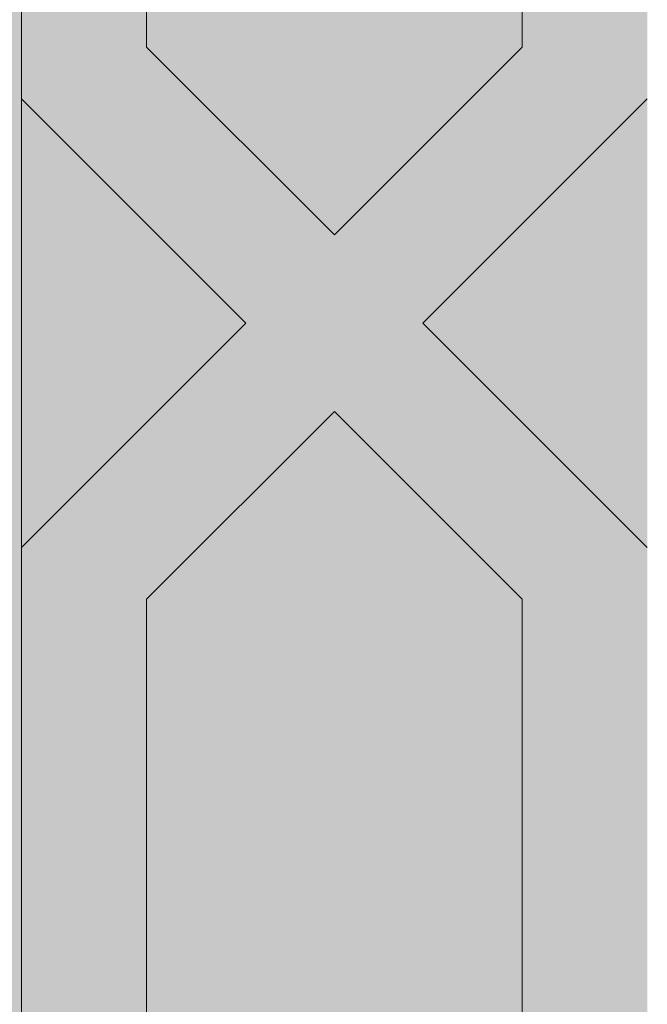
# Model space of a CAD drawing. Units: inches. Extents: x 844 to 2234, y 346 to 1084.
# Tile 70 of 93: x 1997.478 to 1998.757, y 694.327 to 696.335. Entities that reach past the tile are written whole.
import ezdxf

# ---------------------------------------------------------------- set-up
doc = ezdxf.new("R2010")
doc.units = ezdxf.units.IN
doc.header["$MEASUREMENT"] = 0
for name, color, linetype, lineweight in [('A-ANNO-DIMS', 2, 'Continuous', 18), ('furniture', 8, 'Continuous', 18), ('RA-AP-01$0$INT', 35, 'Continuous', 5)]:
    doc.layers.add(name, color=color, linetype=linetype, lineweight=lineweight)
doc.layers.add('RA-AP-01$0$FURN', color=3, linetype='Continuous')
doc.styles.get("Standard").update_dxf_attribs({"font": 'arial.ttf'})
doc.dimstyles.get("Standard").update_dxf_attribs({"dimtxt": 6, "dimasz": 3, "dimexe": 0.18, "dimexo": 0.0625, "dimgap": 0.09, "dimtad": 0, "dimtih": 1, "dimtoh": 1, "dimdec": 1, "dimzin": 0, "dimdsep": 46, "dimlunit": 3, "dimtxsty": 'Standard', "dimblk": 'ARCHTICK', "dimcen": 0.09, "dimadec": 0, "dimazin": 0, "dimtfac": 1, "dimtdec": 1, "dimtofl": 0, "dimtmove": 0, "dimatfit": 3, "dimfxl": 1, "dimtolj": 1, "dimtzin": 0, "dimarcsym": 0})

# ---------------------------------------------------------------- blocks, each defined once
blk = doc.blocks.new('A$C18D01794')
at = {"layer": 'RA-AP-01$0$INT'}
h = blk.add_hatch(color=256, dxfattribs=at)
h.paths.add_polyline_path([(4.355206456958071, -6.156712009588037), (4.355206456958071, -8.056712009588038), (5.455206456958072, -8.056712009588038), (5.455206456958072, -6.156712009588037)])
h.paths.add_polyline_path([(4.405206456958072, -8.006712009588039), (4.405206456958072, -6.206712009588038), (5.405206456958072, -6.206712009588038), (5.405206456958072, -8.006712009588039)], flags=16)
h = blk.add_hatch(color=256, dxfattribs=at)
h.paths.add_polyline_path([(4.469348592586677, -7.07085414521094), (4.505206456958073, -7.03499628085108), (4.505206456958071, -7.106712009593861)])
h.paths.add_polyline_path([(4.455206456960671, -7.084996280832395), (4.476922185709333, -7.106712009588038), (4.433490728198045, -7.106712009588038)])
h.paths.add_polyline_path([(4.405206456958073, -7.034996280813718), (4.441064321339218, -7.070854145206393), (4.40520645695807, -7.106712009576003)])
h.paths.add_polyline_path([(4.425206456989053, -6.911460746921742), (4.455206456990736, -6.881460746929706), (4.485206456989055, -6.911460746937677), (4.48520645696979, -7.026712009590022), (4.455206456965227, -7.056712009584936), (4.425206456969784, -7.026712009579853)])
h.paths.add_polyline_path([(4.505206456958073, -6.831460746955388), (4.505206456958071, -6.903176475661116), (4.469348592616738, -6.867318611308251)])
h.paths.add_polyline_path([(4.425206456964688, -6.707925213036777), (4.455206456964794, -6.677925213027025), (4.485206456964689, -6.707925213017265), (4.485206456983951, -6.823176475683938), (4.455206456990736, -6.853176475686799), (4.425206456983956, -6.823176475689667)])
h.paths.add_polyline_path([(4.425206456974126, -6.504389679118949), (4.455206456959092, -6.474389679124341), (4.485206456974132, -6.504389679129721), (4.485206456993396, -6.619640941768059), (4.45520645699153, -6.649640941779566), (4.425206456993394, -6.619640941791077)])
h.paths.add_polyline_path([(4.46934859260189, -6.663783077416661), (4.505206456958071, -6.627925213048953), (4.505206456958073, -6.699640941761311)])
h.paths.add_polyline_path([(4.405206456958073, -6.627925213005104), (4.441064321354427, -6.663783077389926), (4.405206456958072, -6.699640941797813)])
h.paths.add_polyline_path([(4.405206456958072, -6.424389679139403), (4.441064321333084, -6.460247543502882), (4.405206456958072, -6.496105407889427)])
h.paths.add_polyline_path([(4.469348592580547, -6.460247543498336), (4.505206456958071, -6.424389679109282), (4.505206456958071, -6.496105407864332)])
h.paths.add_polyline_path([(4.425206456957888, -6.300854145208262), (4.45520645695415, -6.270854145221655), (4.485206456959507, -6.300854145217359), (4.48520645695824, -6.416105407863534), (4.455206456954537, -6.44610540787688), (4.425206456957888, -6.416105407889874)])
h.paths.add_polyline_path([(4.425206456957888, -6.226712009591025), (4.471064321332215, -6.226712009591025), (4.425206456957888, -6.272569873980103)])
h.paths.add_polyline_path([(4.499348592575121, -6.226712009591029), (4.636064321343707, -6.226712009591025), (4.666064321342317, -6.256712009589254), (4.636064321340932, -6.286712009591028), (4.499348592588945, -6.286712009591028), (4.469348592591685, -6.256712009584116)])
h.paths.add_polyline_path([(4.680206456964641, -6.270854145214393), (4.716064321337824, -6.306712009588038), (4.644348592591454, -6.306712009588038)])
h.paths.add_polyline_path([(4.644348592588108, -6.206712009588038), (4.716064321341167, -6.206712009588038), (4.680206456964637, -6.242569873964111)])
h.paths.add_polyline_path([(4.724348592586768, -6.226712009589824), (4.861064321340514, -6.226712009589824), (4.891064321340324, -6.256712009589255), (4.861064321340141, -6.286712009589827), (4.724348592587134, -6.286712009589821), (4.694348592586957, -6.256712009589254)])
h.paths.add_polyline_path([(4.905206456964143, -6.270854145212892), (4.941064321338827, -6.306712009588038), (4.869348592589457, -6.306712009588039)])
h.paths.add_polyline_path([(4.869348592586113, -6.206712009588038), (4.941064321342172, -6.206712009588038), (4.905206456964145, -6.242569873965612)])
h.paths.add_polyline_path([(4.949348592587774, -6.226712009589824), (5.086064321341521, -6.226712009589824), (5.116064321341329, -6.256712009589252), (5.08606432134115, -6.286712009589823), (4.949348592588145, -6.286712009589827), (4.919348592587961, -6.256712009589255)])
h.paths.add_polyline_path([(5.130206456963645, -6.270854145214393), (5.166064321336834, -6.306712009588038), (5.094348592590464, -6.306712009588038)])
h.paths.add_polyline_path([(5.094348592587119, -6.206712009588038), (5.166064321340178, -6.206712009588038), (5.130206456963651, -6.242569873964107)])
h.paths.add_polyline_path([(5.174348592584578, -6.226712009591027), (5.311064321353163, -6.226712009591027), (5.341064321336602, -6.256712009584116), (5.31106432133934, -6.286712009591028), (5.174348592587352, -6.286712009591028), (5.144348592585969, -6.256712009589254)])
h.paths.add_polyline_path([(5.325206456968778, -6.300854145217359), (5.355206456974136, -6.270854145221653), (5.385206456970396, -6.300854145208262), (5.385206456970396, -6.416105407889878), (5.355206456973747, -6.44610540787688), (5.325206456970044, -6.416105407863533)])
h.paths.add_polyline_path([(5.339348592596073, -6.226712009591029), (5.385206456970396, -6.226712009591025), (5.385206456970398, -6.272569873980105)])
h.paths.add_polyline_path([(5.325206456954155, -6.504389679129722), (5.355206456969194, -6.474389679124342), (5.38520645695416, -6.504389679118949), (5.385206456934896, -6.619640941791077), (5.355206456936758, -6.649640941779564), (5.325206456934888, -6.619640941768057)])
h.paths.add_polyline_path([(5.305206456958072, -6.424389679097139), (5.341064321347739, -6.460247543498338), (5.305206456958072, -6.496105407876472)])
h.paths.add_polyline_path([(5.369348592595204, -6.460247543502882), (5.40520645695807, -6.42438967915155), (5.405206456958072, -6.496105407877278)])
h.paths.add_polyline_path([(5.405206456958072, -6.627925213017245), (5.405206456958072, -6.69964094178567), (5.369348592573857, -6.663783077389926)])
h.paths.add_polyline_path([(5.305206456958072, -6.62792521303681), (5.341064321326393, -6.663783077416663), (5.305206456958072, -6.69964094177345)])
h.paths.add_polyline_path([(5.325206456963599, -6.707925213017267), (5.355206456963494, -6.677925213027021), (5.385206456963598, -6.707925213036775), (5.385206456944334, -6.823176475689665), (5.355206456937552, -6.853176475686797), (5.325206456944333, -6.823176475683936)])
h.paths.add_polyline_path([(5.305206456958072, -6.831460746943246), (5.341064321311551, -6.867318611308252), (5.305206456958072, -6.903176475673257)])
h.paths.add_polyline_path([(5.325206456939231, -6.911460746937672), (5.355206456937552, -6.881460746929707), (5.385206456939235, -6.911460746921742), (5.385206456958502, -7.026712009579853), (5.355206456963061, -7.056712009584934), (5.3252064569585, -7.026712009590026)])
h.paths.add_polyline_path([(5.404581768715993, -6.832085435167151, 0.001217816984214), (5.405206456958072, -6.832312009593747), (5.405206456958072, -6.90317647569123), (5.369348592563558, -6.867318611308251)])
h.paths.add_polyline_path([(5.36934859258907, -7.070854145206393), (5.40520645695807, -7.034996280825861), (5.405206456958072, -7.106712009563858)])
h.paths.add_polyline_path([(5.355206456967613, -7.084996280832394), (5.376922185730239, -7.106712009588038), (5.333490728218953, -7.106712009588036)])
h.paths.add_polyline_path([(5.30520645695807, -7.034996280838937), (5.341064321341609, -7.070854145210942), (5.305206456958074, -7.106712009606006)])
h = blk.add_hatch(color=256, dxfattribs=at)
h.paths.add_polyline_path([(4.505206456958071, -6.627925213048953), (4.46934859260189, -6.663783077416663), (4.505206456958071, -6.699640941761309), (4.505206456958071, -6.831460746955389), (4.469348592616735, -6.867318611308252), (4.505206456958071, -6.903176475661112), (4.505206456958071, -7.03499628085108), (4.469348592586679, -7.070854145210939), (4.505206456952245, -7.106712009588038), (4.476922185709333, -7.106712009588038), (4.455206456960671, -7.084996280832395), (4.433490728198047, -7.106712009588038), (4.405206456946033, -7.10671200958804), (4.441064321339216, -7.070854145206393), (4.40520645695807, -7.034996280813718), (4.405206456958072, -6.903176475703379), (4.441064321364728, -6.867318611308251), (4.40520645695807, -6.83146074691313), (4.40520645695807, -6.699640941797813), (4.441064321354429, -6.663783077389924), (4.405206456958072, -6.627925213005102), (4.405206456958072, -6.496105407889425), (4.441064321333084, -6.460247543502882), (4.405206456958072, -6.424389679139403), (4.405206456958072, -6.206712009588038), (4.644348592588106, -6.206712009588038), (4.680206456964639, -6.242569873964107), (4.716064321341165, -6.206712009588038), (4.869348592586113, -6.206712009588038), (4.905206456964143, -6.24256987396561), (4.941064321342174, -6.206712009588038), (5.094348592587118, -6.206712009588038), (5.130206456963649, -6.242569873964107), (5.166064321340178, -6.206712009588038), (5.405206456958072, -6.206712009588038), (5.405206456958072, -6.42438967915155), (5.369348592595202, -6.46024754350288), (5.40520645695807, -6.49610540787728), (5.40520645695807, -6.627925213017247), (5.369348592573859, -6.663783077389926), (5.40520645695807, -6.699640941785666), (5.40520645695807, -6.831460746925273), (5.36934859256356, -6.867318611308252), (5.405206456958072, -6.90317647569123), (5.405206456958072, -7.034996280825859), (5.369348592589068, -7.070854145206395), (5.405206456982249, -7.106712009588038), (5.376922185730244, -7.106712009588038), (5.355206456967613, -7.084996280832397), (5.333490728218955, -7.106712009588036), (5.305206456976043, -7.106712009588035), (5.341064321341609, -7.07085414521094), (5.305206456958072, -7.034996280838935), (5.305206456958072, -6.90317647567326), (5.34106432131155, -6.867318611308252), (5.305206456958072, -6.831460746943244), (5.30520645695807, -6.699640941773452), (5.341064321326395, -6.663783077416663), (5.305206456958072, -6.627925213036814), (5.305206456958072, -6.496105407876472), (5.341064321347738, -6.46024754349834), (5.305206456958072, -6.424389679097137), (5.30520645695807, -6.306712009588038), (5.166064321336834, -6.306712009588038), (5.130206456963647, -6.270854145214393), (5.094348592590464, -6.306712009588038), (4.941064321338827, -6.306712009588036), (4.905206456964145, -6.270854145212892), (4.869348592589459, -6.306712009588038), (4.716064321337822, -6.306712009588036), (4.680206456964641, -6.270854145214393), (4.644348592591453, -6.306712009588038), (4.505206456958071, -6.306712009588038), (4.505206456958071, -6.424389679109282), (4.469348592580545, -6.460247543498338), (4.505206456958071, -6.496105407864328)])
h.paths.add_polyline_path([(4.485206456974132, -6.504389679129722), (4.45520645695909, -6.474389679124341), (4.425206456974128, -6.504389679118945), (4.425206456993394, -6.619640941791079), (4.45520645699153, -6.649640941779566), (4.485206456993396, -6.619640941768059)], flags=16)
h.paths.add_polyline_path([(4.455206456954537, -6.44610540787688), (4.485206456958242, -6.416105407863534), (4.48520645695951, -6.30085414521736), (4.45520645695415, -6.270854145221653), (4.425206456957888, -6.300854145208264), (4.425206456957888, -6.41610540788988)], flags=16)
h.paths.add_polyline_path([(4.455206456964794, -6.677925213027025), (4.42520645696469, -6.707925213036777), (4.425206456983954, -6.82317647568967), (4.455206456990734, -6.853176475686797), (4.485206456983953, -6.823176475683936), (4.485206456964687, -6.707925213017265)], flags=16)
h.paths.add_polyline_path([(4.499348592588947, -6.286712009591028), (4.636064321340932, -6.286712009591028), (4.666064321342317, -6.256712009589254), (4.636064321343707, -6.226712009591027), (4.499348592575121, -6.226712009591029), (4.469348592591685, -6.256712009584118)], flags=16)
h.paths.add_polyline_path([(4.425206456957888, -6.272569873980103), (4.471064321332215, -6.226712009591025), (4.425206456957888, -6.226712009591025)], flags=16)
h.paths.add_polyline_path([(4.455206456990734, -6.881460746929709), (4.425206456989053, -6.91146074692174), (4.425206456969784, -7.026712009579853), (4.455206456965226, -7.056712009584932), (4.485206456969787, -7.026712009590026), (4.485206456989053, -6.911460746937672)], flags=16)
h.paths.add_polyline_path([(4.72434859258714, -6.286712009589821), (4.861064321340141, -6.286712009589829), (4.891064321340324, -6.256712009589254), (4.861064321340513, -6.226712009589823), (4.724348592586768, -6.226712009589823), (4.694348592586956, -6.256712009589254)], flags=16)
h.paths.add_polyline_path([(4.919348592587961, -6.256712009589254), (4.949348592588145, -6.286712009589827), (5.08606432134115, -6.286712009589823), (5.116064321341327, -6.256712009589254), (5.086064321341519, -6.226712009589824), (4.949348592587774, -6.226712009589824)], flags=16)
h.paths.add_polyline_path([(5.144348592585967, -6.256712009589254), (5.174348592587358, -6.286712009591028), (5.311064321339338, -6.286712009591028), (5.3410643213366, -6.256712009584118), (5.311064321353163, -6.226712009591029), (5.174348592584576, -6.226712009591027)], flags=16)
h.paths.add_polyline_path([(5.32520645693489, -6.619640941768055), (5.355206456936755, -6.649640941779566), (5.385206456934894, -6.619640941791079), (5.38520645695416, -6.504389679118949), (5.355206456969194, -6.474389679124341), (5.325206456954153, -6.504389679129724)], flags=16)
h.paths.add_polyline_path([(5.325206456970042, -6.416105407863534), (5.355206456973747, -6.44610540787688), (5.385206456970398, -6.416105407889876), (5.385206456970398, -6.30085414520826), (5.355206456974136, -6.270854145221653), (5.325206456968778, -6.30085414521736)], flags=16)
h.paths.add_polyline_path([(5.325206456963599, -6.707925213017265), (5.325206456944333, -6.823176475683936), (5.355206456937552, -6.853176475686797), (5.385206456944332, -6.823176475689667), (5.385206456963596, -6.707925213036773), (5.355206456963492, -6.677925213027027)], flags=16)
h.paths.add_polyline_path([(5.32520645693923, -6.911460746937674), (5.3252064569585, -7.026712009590026), (5.355206456963062, -7.056712009584934), (5.3852064569585, -7.026712009579853), (5.385206456939234, -6.911460746921738), (5.355206456937552, -6.881460746929707)], flags=16)
h.paths.add_polyline_path([(5.339348592596071, -6.226712009591029), (5.385206456970398, -6.272569873980103), (5.385206456970396, -6.226712009591027)], flags=16)
for p, q in [((5.32520645693489, -6.619640941768059), (5.325206456954155, -6.504389679129722)), ((5.385206456934892, -6.619640941791081), (5.385206456954159, -6.504389679118947)), ((5.32520645693489, -6.619640941768059), (5.355206456936756, -6.649640941779566)), ((5.385206456934892, -6.619640941791081), (5.355206456936756, -6.649640941779566)), ((5.305206456939818, -6.627925213018556), (5.341064321310754, -6.663783077401021)), ((5.405206456939818, -6.627925213035499), (5.369348592558215, -6.663783077405568)), ((5.305206456959569, -6.699640941771955), (5.341064321342035, -6.663783077401022)), ((5.405206456959569, -6.699640941787167), (5.369348592589498, -6.663783077405566)), ((5.325206456963599, -6.707925213017265), (5.35520645696349, -6.677925213027025)), ((5.385206456963598, -6.707925213036777), (5.35520645696349, -6.677925213027025)), ((5.325206456944333, -6.823176475683936), (5.325206456963599, -6.707925213017265)), ((5.385206456944332, -6.823176475689667), (5.385206456963598, -6.707925213036777))]:
    blk.add_line(p, q, dxfattribs=at)
blk.add_lwpolyline([(5.405206456958072, -7.106712009588038), (5.405206456958072, -6.206712009588038)], dxfattribs=at)
blk = doc.blocks.new('A$C5D2F253E')
at = {"layer": 'RA-AP-01$0$FURN', "xscale": -0.7999999999883585, "yscale": 0.7999999999883585, "zscale": 0.8, "rotation": 90}
blk.add_blockref('A$C18D01794', (-5.687757199772477, 4.75791982714071), dxfattribs=at)
blk = doc.blocks.new('_ArchTick')
at = {"color": 0, "linetype": 'ByBlock', "const_width": 0.15}
blk.add_lwpolyline([(-0.5, -0.5), (0.5, 0.5)], dxfattribs=at)
blk = doc.blocks.new('*D121')
at = {"layer": 'A-ANNO-DIMS', "color": 0, "lineweight": -2, "transparency": 16777216}
for p, q in [((2030.271987351997, 734.262611118704), (2040.245275089302, 734.262611118704)), ((2040.065275089302, 734.262611118704), (2040.065275089302, 704.6043509484256)), ((2040.065275089302, 668.557359536674), (2040.065275089302, 698.2156197069523)), ((2030.271987351997, 668.557359536674), (2040.245275089302, 668.557359536674))]:
    blk.add_line(p, q, dxfattribs=at)
at = {"layer": 'Defpoints', "color": 0, "transparency": 16777216}
for p in [(2030.209487351997, 734.262611118704), (2040.065275089302, 734.262611118704), (2030.209487351997, 668.557359536674)]:
    blk.add_point(p, dxfattribs=at)
at = {"layer": 'A-ANNO-DIMS', "color": 0, "lineweight": -2, "transparency": 16777216, "xscale": 3, "yscale": 3, "zscale": 3}
for p, rotation in [((2040.065275089302, 734.262611118704), 90), ((2040.065275089302, 668.557359536674), 270)]:
    blk.add_blockref('_ArchTick', p, dxfattribs=dict(at, rotation=rotation))
at = {"layer": 'A-ANNO-DIMS', "color": 0, "transparency": 16777216, "insert": (2040.065275089302, 701.4099853276883), "char_height": 6, "attachment_point": 5}
blk.add_mtext('\\A1;LOUNGE SET 5\'-5 1/2" TYP.', dxfattribs=at)

msp = doc.modelspace()

# ---------------------------------------------------------------- block references
at = {"layer": 'furniture', "xscale": -15.94108302203742, "yscale": 15.94108302203742, "zscale": 15.94108302203742, "rotation": 270}
msp.add_blockref('A$C5D2F253E', (1990.567271852805, 701.4028671565849), dxfattribs=at)

# ---------------------------------------------------------------- dimensions: what is measured, and where the dimension line sits
at = {"layer": 'A-ANNO-DIMS'}
dim = msp.add_linear_dim(base=(2040.065275089302, 734.262611118704), p1=(2030.209487351996, 668.5573595366737), p2=(2030.209487351996, 734.2626111187037), angle=90, text='LOUNGE SET <> TYP.', dimstyle='Standard', override={"dimdec": 1, "dimlfac": 1, "dimrnd": 0, "dimzin": 1, "dimdsep": 46, "dimlunit": 4, "dimfrac": 2}, dxfattribs=at)
dim.commit()
dim.dimension.update_dxf_attribs({"geometry": '*D121', "text_midpoint": (2040.065275089302, 701.4099853276883)})

doc.saveas('drawing.dxf')
